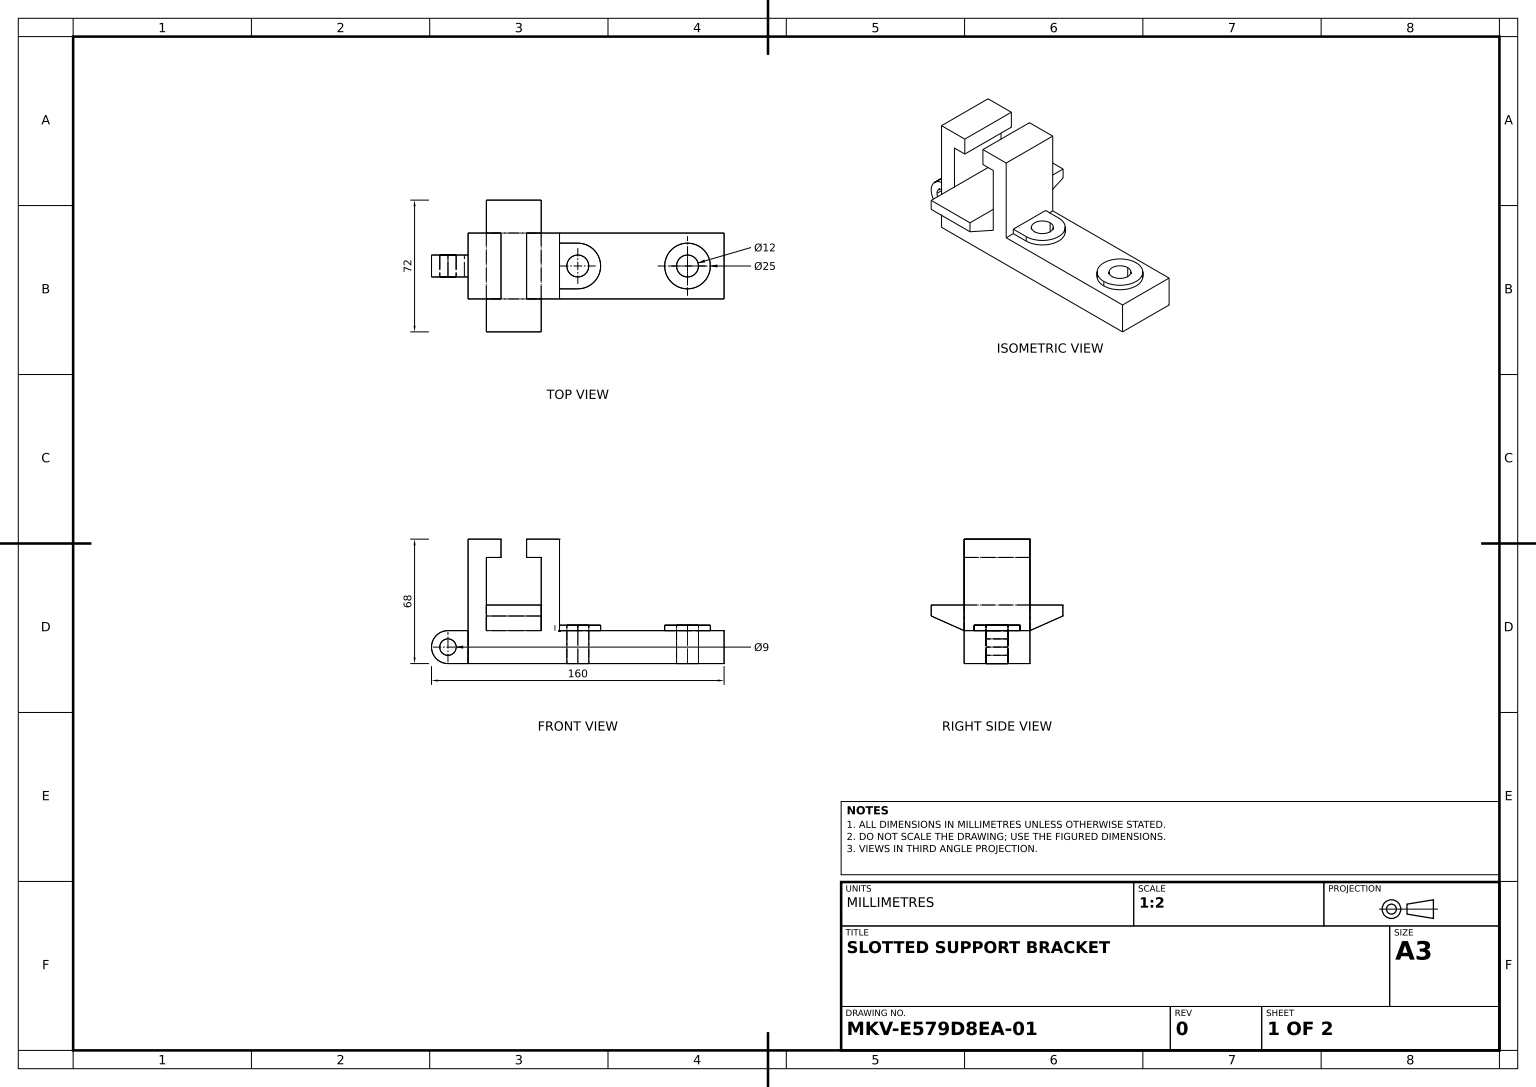
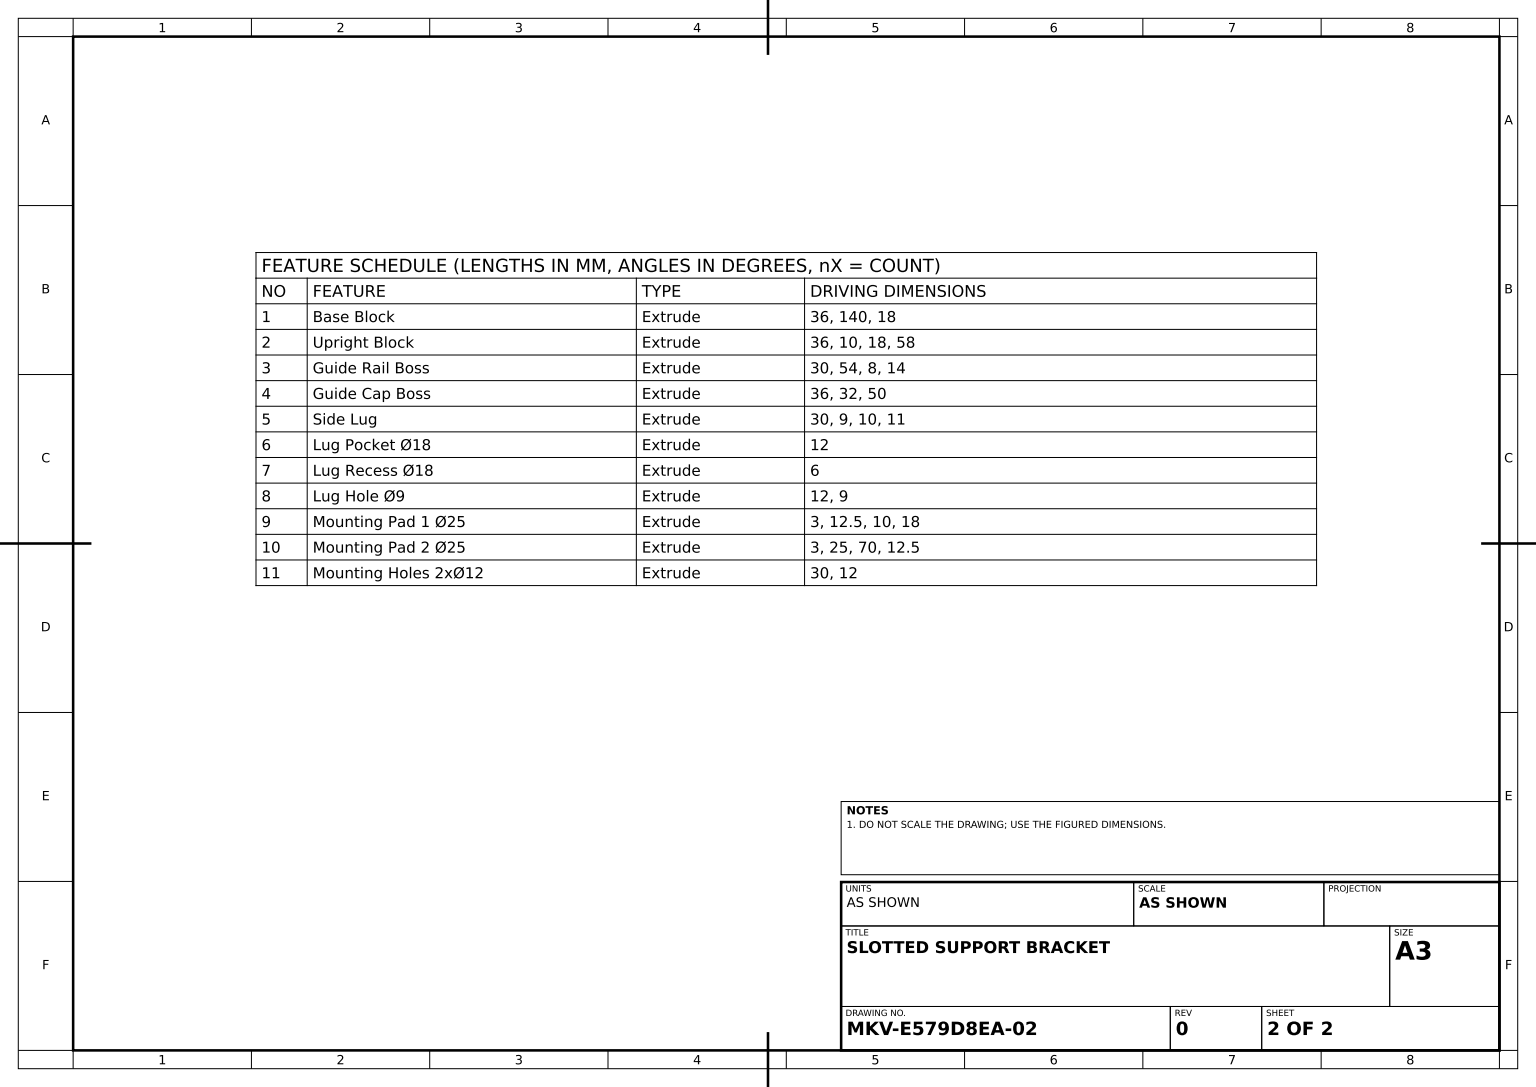
from build123d import *

# Parameters (mm, degrees)
BASE_PROFILE_SKETCH_W      = 140
BASE_PROFILE_SKETCH_H      = 18
BASE_BLOCK_DEPTH           = 36
UPRIGHT_BLOCK_DEPTH        = 36
GUIDE_RAIL_BOSS_DEPTH      = 30
GUIDE_CAP_BOSS_DEPTH       = 36
SIDE_LUG_DEPTH             = 30
LUG_POCKET_18_DEPTH        = 12
LUG_START                  = -6
LUG_RECESS_18_DEPTH        = 6
LUG_HOLE_SKETCH_R          = 4.5
LUG_HOLE_9_DEPTH           = 12
MOUNTING_PAD_1_25_DEPTH    = 3
MOUNTING_PAD_2_SKETCH_R    = 12.5
MOUNTING_PAD_2_25_DEPTH    = 3
MOUNTING_HOLES_SKETCH_R    = 6
MOUNTING_HOLES_2X_12_DEPTH = 30


with BuildPart() as part:
    # Base Profile Sketch → Base Block (new body)
    with BuildSketch(Plane.XY):
        with Locations((70, 9)):
            Rectangle(BASE_PROFILE_SKETCH_W, BASE_PROFILE_SKETCH_H)
    extrude(amount=BASE_BLOCK_DEPTH)

    # Upright Profile Sketch → Upright Block (add)
    with BuildSketch(Plane.XY.offset(36)):
        Polygon((0, 18), (0, 68), (18, 68), (18, 58), (10, 58), (10, 18), align=None)
    extrude(amount=-UPRIGHT_BLOCK_DEPTH)

    # Guide Rail Sketch → Guide Rail Boss (add)
    with BuildSketch(Plane(origin=(10, 0, 0), x_dir=(0, 0, -1), z_dir=(1, 0, 0))):
        Polygon((-18, 32), (18, 32), (18, 26), (0, 18), (-18, 18), (-36, 18), (-54, 26), (-54, 32), align=None)
    extrude(amount=GUIDE_RAIL_BOSS_DEPTH)

    # Guide Cap Sketch → Guide Cap Boss (add)
    with BuildSketch(Plane(origin=(0, 0, 0), x_dir=(-1, 0, 0), z_dir=(0, 0, -1))):
        Polygon((-40, 18), (-50, 18), (-50, 68), (-32, 68), (-32, 58), (-40, 58), align=None)
    extrude(amount=-GUIDE_CAP_BOSS_DEPTH)

    # Side Lug Sketch → Side Lug (add)
    with BuildSketch(Plane(origin=(0, 0, 0), x_dir=(-1, 0, 0), z_dir=(0, 0, -1))):
        with BuildLine():
            Line((0, 0), (0, 18))
            Line((0, 18), (10, 18))
            Line((10, 18), (11, 18))
            ThreePointArc((11, 18), (20, 9), (11, 0))
            Line((11, 0), (0, 0))
        make_face()
    extrude(amount=-SIDE_LUG_DEPTH)

    # Lug Pocket Sketch → Lug Pocket Ø18 (cut)
    with BuildSketch(Plane(origin=(0, 0, 0), x_dir=(-1, 0, 0), z_dir=(0, 0, -1))):
        with BuildLine():
            Line((0, 18), (11, 18))
            ThreePointArc((11, 18), (20, 9), (11, 0))
            Line((11, 0), (0, 0))
            Line((0, 0), (0, 18))
        make_face()
    extrude(amount=-LUG_POCKET_18_DEPTH, mode=Mode.SUBTRACT)

    # Lug Recess Sketch → Lug Recess Ø18 (cut)
    with BuildSketch(Plane.XY.offset(30).offset(LUG_START)):
        with BuildLine():
            Line((0, 18), (-11, 18))
            ThreePointArc((-11, 18), (-20, 9), (-11, 0))
            Line((-11, 0), (0, 0))
            Line((0, 0), (0, 18))
        make_face()
    extrude(amount=LUG_RECESS_18_DEPTH, mode=Mode.SUBTRACT)

    # Lug Hole Sketch → Lug Hole Ø9 (cut)
    with BuildSketch(Plane.XY.offset(24)):
        with Locations((-11, 9)):
            Circle(LUG_HOLE_SKETCH_R)
    extrude(amount=-LUG_HOLE_9_DEPTH, mode=Mode.SUBTRACT)

    # Mounting Pad 1 Sketch → Mounting Pad 1 Ø25 (add)
    with BuildSketch(Plane(origin=(0, 18, 0), x_dir=(1, 0, 0), z_dir=(0, 1, 0))):
        with BuildLine():
            Line((60, -5.5), (50, -5.5))
            Line((50, -5.5), (50, -30.5))
            Line((50, -30.5), (60, -30.5))
            ThreePointArc((60, -30.5), (72.5, -18), (60, -5.5))
        make_face()
    extrude(amount=MOUNTING_PAD_1_25_DEPTH)

    # Mounting Pad 2 Sketch → Mounting Pad 2 Ø25 (add)
    with BuildSketch(Plane(origin=(0, 18, 0), x_dir=(1, 0, 0), z_dir=(0, 1, 0))):
        with Locations(Location((120, -18, 0), (0, 0, 90))):
            Circle(MOUNTING_PAD_2_SKETCH_R)
    extrude(amount=MOUNTING_PAD_2_25_DEPTH)

    # Mounting Holes Sketch → Mounting Holes 2xØ12 (cut)
    with BuildSketch(Plane(origin=(0, 21, 0), x_dir=(1, 0, 0), z_dir=(0, 1, 0))):
        with Locations(Location((120, -18, 0), (0, 0, 270))):
            Circle(MOUNTING_HOLES_SKETCH_R)
        with Locations(Location((60, -18, 0), (0, 0, 270))):
            Circle(MOUNTING_HOLES_SKETCH_R)
    extrude(amount=-MOUNTING_HOLES_2X_12_DEPTH, mode=Mode.SUBTRACT)


solid = part.part
